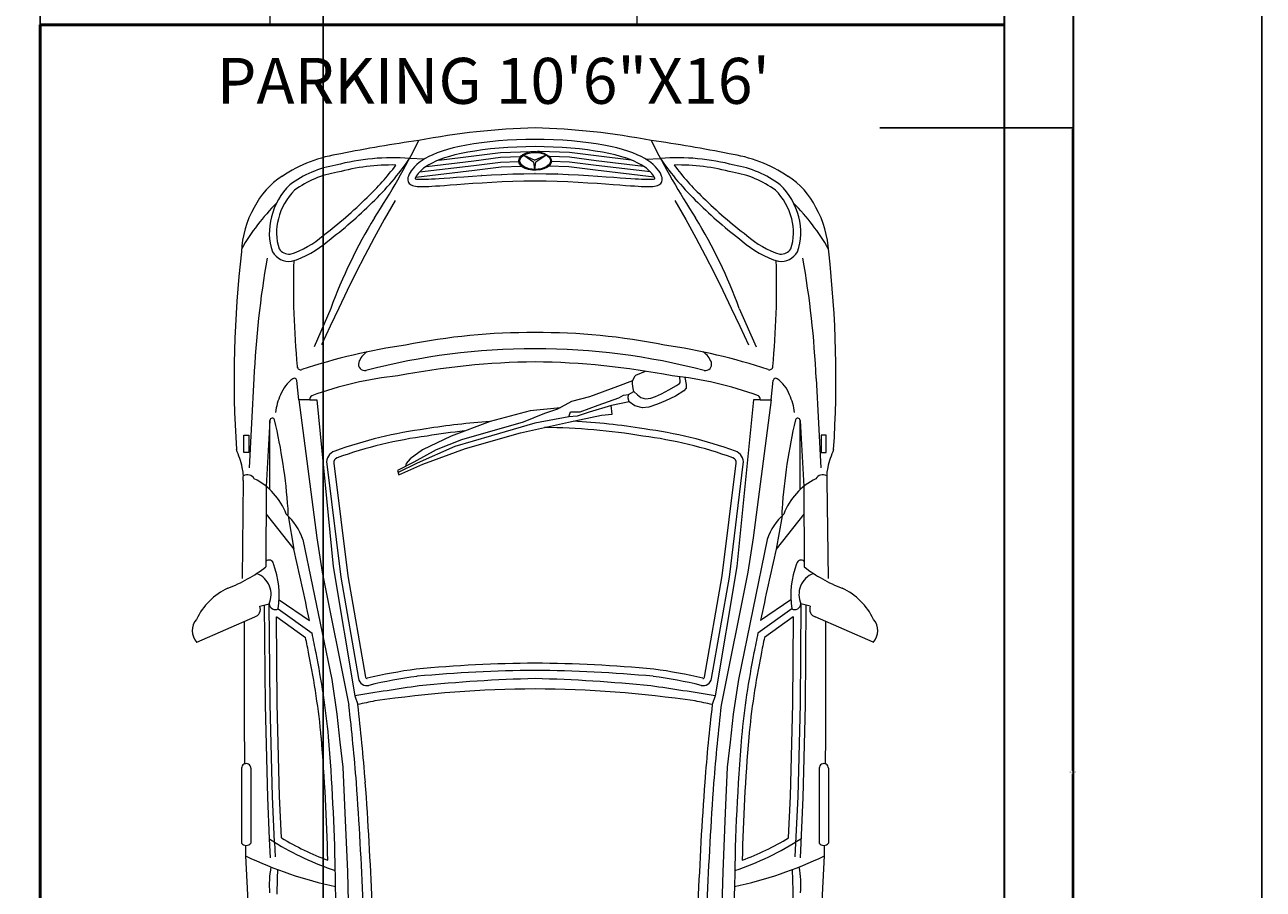
# Model space of a CAD drawing. Units: inches. Extents: x 8049 to 8459, y 820 to 1350.
# Tile 21 of 25: x 8297 to 8459, y 933 to 1046. Entities that reach past the tile are written whole.
import ezdxf

# ---------------------------------------------------------------- set-up
doc = ezdxf.new("R2010")
doc.units = ezdxf.units.IN
doc.header["$MEASUREMENT"] = 0
for name, color, linetype, lineweight in [('A-ANNO-DIMS', 2, 'Continuous', 18), ('A-AREA-IDEN', 7, 'Continuous', 25), ('A-GLAZ', 4, 'Continuous', 18), ('A-WALL', 7, 'Continuous', 50), ('C-PKNG-VEH', 8, 'Continuous', 13), ('C-SITE-WALL', 7, 'Continuous', 35)]:
    doc.layers.add(name, color=color, linetype=linetype, lineweight=lineweight)
doc.styles.get("Standard").update_dxf_attribs({"font": 'arial.ttf'})
doc.dimstyles.get("Standard").update_dxf_attribs({"dimtxt": 0.18, "dimasz": 0.18, "dimexe": 0.18, "dimexo": 0.0625, "dimgap": 0.09, "dimtad": 0, "dimtih": 1, "dimtoh": 1, "dimdec": 4, "dimzin": 0, "dimdsep": 46, "dimtxsty": 'Standard', "dimcen": 0.09, "dimadec": 0, "dimazin": 0, "dimtfac": 1, "dimtdec": 4, "dimtofl": 0, "dimtmove": 0, "dimatfit": 3, "dimfxl": 1, "dimtolj": 1, "dimtzin": 0, "dimarcsym": 0})

# ---------------------------------------------------------------- blocks, each defined once
blk = doc.blocks.new('A$C27D64469')
for p, q in [((-0.156, -0.4453), (-0.1764, -0.4487)), ((-0.1343, -0.4422), (-0.156, -0.4453)), ((-0.1114, -0.4395), (-0.1343, -0.4422)), ((-0.0875, -0.4373), (-0.1114, -0.4395)), ((-0.0629, -0.4354), (-0.0875, -0.4373)), ((-0.0377, -0.4341), (-0.0629, -0.4354)), ((-0.0122, -0.4333), (-0.0377, -0.4341)), ((0.0136, -0.433), (-0.0122, -0.4333)), ((0.0393, -0.4333), (0.0136, -0.433)), ((0.0649, -0.4341), (0.0393, -0.4333)), ((0.0901, -0.4354), (0.0649, -0.4341)), ((0.1147, -0.4373), (0.0901, -0.4354)), ((0.1385, -0.4395), (0.1147, -0.4373)), ((0.1614, -0.4422), (0.1385, -0.4395)), ((0.1832, -0.4453), (0.1614, -0.4422)), ((0.2036, -0.4487), (0.1832, -0.4453)), ((-0.2693, -0.4753), (-0.2803, -0.4806)), ((-0.2571, -0.4703), (-0.2693, -0.4753)), ((-0.2436, -0.4655), (-0.2571, -0.4703)), ((-0.253, -0.4902), (-0.1557, -0.4786)), ((-0.2289, -0.4609), (-0.2436, -0.4655)), ((-0.2128, -0.4566), (-0.2289, -0.4609)), ((-0.208, -0.476), (-0.2233, -0.4801)), ((-0.1954, -0.4525), (-0.2128, -0.4566)), ((-0.1912, -0.4721), (-0.208, -0.476)), ((-0.1764, -0.4487), (-0.1954, -0.4525)), ((-0.1728, -0.4684), (-0.1912, -0.4721)), ((-0.153, -0.4651), (-0.1728, -0.4684)), ((-0.1557, -0.4786), (-0.0819, -0.4693)), ((-0.1317, -0.4621), (-0.153, -0.4651)), ((-0.1093, -0.4594), (-0.1317, -0.4621)), ((-0.0858, -0.4572), (-0.1093, -0.4594)), ((-0.0616, -0.4554), (-0.0858, -0.4572)), ((-0.0819, -0.4693), (0.0012, -0.4665)), ((-0.0369, -0.4541), (-0.0616, -0.4554)), ((-0.0117, -0.4533), (-0.0369, -0.4541)), ((-0.0174, -0.4766), (0.0132, -0.4908)), ((-0.0174, -0.4766), (0.0101, -0.4961)), ((0.0136, -0.453), (-0.0117, -0.4533)), ((0.0012, -0.4665), (0.0067, -0.4665)), ((0.0445, -0.4762), (0.0132, -0.4908)), ((0.0389, -0.4533), (0.0136, -0.453)), ((0.0445, -0.4762), (0.0162, -0.4961)), ((0.0259, -0.4665), (0.0204, -0.4665)), ((0.109, -0.4693), (0.0259, -0.4665)), ((0.064, -0.4541), (0.0389, -0.4533)), ((0.0888, -0.4554), (0.064, -0.4541)), ((0.113, -0.4572), (0.0888, -0.4554)), ((0.1828, -0.4786), (0.109, -0.4693)), ((0.1364, -0.4594), (0.113, -0.4572)), ((0.1588, -0.4621), (0.1364, -0.4594)), ((0.1801, -0.4651), (0.1588, -0.4621)), ((0.2, -0.4684), (0.1801, -0.4651)), ((0.2801, -0.4902), (0.1828, -0.4786)), ((0.2183, -0.4721), (0.2, -0.4684)), ((0.2225, -0.4525), (0.2036, -0.4487)), ((0.2351, -0.476), (0.2183, -0.4721)), ((0.24, -0.4566), (0.2225, -0.4525)), ((0.2505, -0.4801), (0.2351, -0.476)), ((0.2561, -0.4609), (0.24, -0.4566)), ((0.2708, -0.4655), (0.2561, -0.4609)), ((0.2842, -0.4703), (0.2708, -0.4655)), ((0.2964, -0.4753), (0.2842, -0.4703)), ((0.3075, -0.4806), (0.2964, -0.4753)), ((-0.2923, -0.4873), (-0.3337, -0.4857)), ((-0.3248, -0.514), (-0.329, -0.5195)), ((-0.3198, -0.5085), (-0.3248, -0.514)), ((-0.3138, -0.5028), (-0.3198, -0.5085)), ((-0.307, -0.4972), (-0.3138, -0.5028)), ((-0.2991, -0.4915), (-0.307, -0.4972)), ((-0.306, -0.5231), (-0.1557, -0.5051)), ((-0.2947, -0.513), (-0.3006, -0.5178)), ((-0.2902, -0.486), (-0.2991, -0.4915)), ((-0.288, -0.5082), (-0.2947, -0.513)), ((-0.2803, -0.4806), (-0.2902, -0.486)), ((-0.2883, -0.5077), (-0.2883, -0.5077)), ((-0.2801, -0.5033), (-0.288, -0.5082)), ((-0.287, -0.5076), (-0.1557, -0.4919)), ((-0.2712, -0.4984), (-0.2801, -0.5033)), ((-0.2612, -0.4936), (-0.2712, -0.4984)), ((-0.2499, -0.489), (-0.2612, -0.4936)), ((-0.2373, -0.4844), (-0.2499, -0.489)), ((-0.2233, -0.4801), (-0.2373, -0.4844)), ((-0.1557, -0.4919), (-0.0819, -0.4825)), ((-0.1557, -0.5051), (-0.0819, -0.4958)), ((-0.154, -0.5181), (-0.0802, -0.5088)), ((-0.0819, -0.4825), (-0.0265, -0.4807)), ((-0.0819, -0.4958), (-0.0315, -0.4941)), ((-0.0802, -0.5088), (-0.0242, -0.5069)), ((0.0133, -0.5159), (0.0101, -0.4961)), ((0.0133, -0.5159), (0.0162, -0.4961)), ((0.1074, -0.5088), (0.0513, -0.5069)), ((0.109, -0.4825), (0.0537, -0.4807)), ((0.109, -0.4958), (0.0586, -0.4941)), ((0.1811, -0.5181), (0.1074, -0.5088)), ((0.1828, -0.4919), (0.109, -0.4825)), ((0.1828, -0.5051), (0.109, -0.4958)), ((0.3141, -0.5076), (0.1828, -0.4919)), ((0.3332, -0.5231), (0.1828, -0.5051)), ((0.2644, -0.4844), (0.2505, -0.4801)), ((0.277, -0.489), (0.2644, -0.4844)), ((0.2883, -0.4936), (0.277, -0.489)), ((0.2984, -0.4984), (0.2883, -0.4936)), ((0.3073, -0.5033), (0.2984, -0.4984)), ((0.3151, -0.5082), (0.3073, -0.5033)), ((0.3174, -0.486), (0.3075, -0.4806)), ((0.3219, -0.513), (0.3151, -0.5082)), ((0.3262, -0.4915), (0.3174, -0.486)), ((0.3195, -0.4873), (0.3609, -0.4857)), ((0.3277, -0.5178), (0.3219, -0.513)), ((0.3341, -0.4972), (0.3262, -0.4915)), ((0.341, -0.5028), (0.3341, -0.4972)), ((0.3469, -0.5085), (0.341, -0.5028)), ((0.352, -0.514), (0.3469, -0.5085)), ((0.3562, -0.5195), (0.352, -0.514)), ((-0.3381, -0.5386), (-0.3386, -0.5425)), ((-0.3386, -0.5425), (-0.3385, -0.5462)), ((-0.3385, -0.5462), (-0.3378, -0.5495)), ((-0.3369, -0.5343), (-0.3381, -0.5386)), ((-0.3351, -0.5296), (-0.3369, -0.5343)), ((-0.3324, -0.5247), (-0.3351, -0.5296)), ((-0.329, -0.5195), (-0.3324, -0.5247)), ((-0.318, -0.5407), (-0.3183, -0.5417)), ((-0.3183, -0.5417), (-0.3172, -0.542)), ((-0.3169, -0.5381), (-0.318, -0.5407)), ((-0.3172, -0.542), (-0.3144, -0.5426)), ((-0.3152, -0.5348), (-0.3169, -0.5381)), ((-0.3166, -0.5376), (-0.154, -0.5181)), ((-0.3127, -0.5311), (-0.3152, -0.5348)), ((-0.3144, -0.5426), (-0.3108, -0.543)), ((-0.3095, -0.5269), (-0.3127, -0.5311)), ((-0.3108, -0.543), (-0.3063, -0.5433)), ((-0.3055, -0.5225), (-0.3095, -0.5269)), ((-0.3063, -0.5433), (-0.3012, -0.5434)), ((-0.3006, -0.5178), (-0.3055, -0.5225)), ((-0.3012, -0.5434), (-0.2953, -0.5434)), ((-0.2953, -0.5434), (-0.2888, -0.5433)), ((-0.2888, -0.5433), (-0.2815, -0.543)), ((-0.2815, -0.543), (-0.2731, -0.5425)), ((-0.2731, -0.5425), (-0.2632, -0.5419)), ((-0.2632, -0.5419), (-0.2517, -0.5411)), ((-0.2517, -0.5411), (-0.2382, -0.5402)), ((-0.2382, -0.5402), (-0.2225, -0.539)), ((-0.2225, -0.539), (-0.2042, -0.5376)), ((-0.2042, -0.5376), (-0.1833, -0.5361)), ((-0.1832, -0.5361), (-0.1598, -0.5344)), ((-0.1597, -0.5344), (-0.1342, -0.5327)), ((-0.1341, -0.5327), (-0.1069, -0.5311)), ((-0.1067, -0.5311), (-0.0781, -0.5297)), ((-0.0779, -0.5297), (-0.0482, -0.5285)), ((-0.048, -0.5285), (-0.0176, -0.5278)), ((-0.0475, -0.5485), (-0.0171, -0.5478)), ((-0.0173, -0.5278), (0.0134, -0.5275)), ((-0.0171, -0.5478), (0.0136, -0.5475)), ((0.0136, -0.5475), (0.0443, -0.5478)), ((0.0138, -0.5275), (0.0444, -0.5278)), ((0.0443, -0.5478), (0.0746, -0.5485)), ((0.0448, -0.5278), (0.0751, -0.5285)), ((0.0754, -0.5285), (0.105, -0.5297)), ((0.1052, -0.5297), (0.1339, -0.5311)), ((0.134, -0.5311), (0.1612, -0.5327)), ((0.1614, -0.5327), (0.1869, -0.5344)), ((0.3438, -0.5376), (0.1811, -0.5181)), ((0.187, -0.5344), (0.2103, -0.5361)), ((0.2104, -0.5361), (0.2314, -0.5376)), ((0.2314, -0.5376), (0.2496, -0.539)), ((0.2496, -0.539), (0.2653, -0.5402)), ((0.2653, -0.5402), (0.2788, -0.5411)), ((0.2788, -0.5411), (0.2904, -0.5419)), ((0.2904, -0.5419), (0.3002, -0.5425)), ((0.3002, -0.5425), (0.3087, -0.543)), ((0.3087, -0.543), (0.316, -0.5433)), ((0.316, -0.5433), (0.3225, -0.5434)), ((0.3225, -0.5434), (0.3283, -0.5434)), ((0.3326, -0.5225), (0.3277, -0.5178)), ((0.3283, -0.5434), (0.3335, -0.5433)), ((0.3367, -0.5269), (0.3326, -0.5225)), ((0.3335, -0.5433), (0.3379, -0.543)), ((0.3399, -0.5311), (0.3367, -0.5269)), ((0.3379, -0.543), (0.3416, -0.5426)), ((0.3423, -0.5348), (0.3399, -0.5311)), ((0.3416, -0.5426), (0.3444, -0.542)), ((0.3441, -0.5381), (0.3423, -0.5348)), ((0.3451, -0.5407), (0.3441, -0.5381)), ((0.3444, -0.542), (0.3454, -0.5417)), ((0.3454, -0.5417), (0.3451, -0.5407)), ((0.3596, -0.5247), (0.3562, -0.5195)), ((0.3622, -0.5296), (0.3596, -0.5247)), ((0.3641, -0.5343), (0.3622, -0.5296)), ((0.3653, -0.5386), (0.3641, -0.5343)), ((0.3649, -0.5495), (0.3656, -0.5462)), ((0.3658, -0.5425), (0.3653, -0.5386)), ((0.3656, -0.5462), (0.3658, -0.5425)), ((-0.3378, -0.5495), (-0.3364, -0.5524)), ((-0.3364, -0.5524), (-0.3345, -0.5549)), ((-0.3345, -0.5549), (-0.3321, -0.5571)), ((-0.3321, -0.5571), (-0.3292, -0.5589)), ((-0.3292, -0.5589), (-0.3258, -0.5604)), ((-0.3258, -0.5604), (-0.3219, -0.5615)), ((-0.3219, -0.5615), (-0.3175, -0.5623)), ((-0.3175, -0.5623), (-0.3126, -0.5629)), ((-0.3126, -0.5629), (-0.3072, -0.5633)), ((-0.3072, -0.5633), (-0.3014, -0.5634)), ((-0.3014, -0.5634), (-0.2951, -0.5634)), ((-0.2951, -0.5634), (-0.2882, -0.5633)), ((-0.2882, -0.5633), (-0.2806, -0.563)), ((-0.2806, -0.563), (-0.272, -0.5625)), ((-0.272, -0.5625), (-0.2619, -0.5619)), ((-0.2619, -0.5619), (-0.2503, -0.5611)), ((-0.2503, -0.5611), (-0.2367, -0.5601)), ((-0.2367, -0.5601), (-0.221, -0.559)), ((-0.221, -0.559), (-0.2027, -0.5576)), ((-0.2027, -0.5576), (-0.1818, -0.556)), ((-0.1818, -0.556), (-0.1584, -0.5544)), ((-0.1584, -0.5544), (-0.1329, -0.5527)), ((-0.1329, -0.5527), (-0.1057, -0.5511)), ((-0.1057, -0.5511), (-0.0771, -0.5496)), ((-0.0771, -0.5496), (-0.0475, -0.5485)), ((0.0746, -0.5485), (0.1043, -0.5496)), ((0.1043, -0.5496), (0.1329, -0.5511)), ((0.1329, -0.5511), (0.1601, -0.5527)), ((0.1601, -0.5527), (0.1855, -0.5544)), ((0.1855, -0.5544), (0.2089, -0.556)), ((0.2089, -0.556), (0.2299, -0.5576)), ((0.2299, -0.5576), (0.2481, -0.559)), ((0.2481, -0.559), (0.2639, -0.5601)), ((0.2639, -0.5601), (0.2775, -0.5611)), ((0.2775, -0.5611), (0.2891, -0.5619)), ((0.2891, -0.5619), (0.2991, -0.5625)), ((0.2991, -0.5625), (0.3078, -0.563)), ((0.3078, -0.563), (0.3154, -0.5633)), ((0.3154, -0.5633), (0.3222, -0.5634)), ((0.3222, -0.5634), (0.3285, -0.5634)), ((0.3285, -0.5634), (0.3344, -0.5633)), ((0.3344, -0.5633), (0.3398, -0.5629)), ((0.3398, -0.5629), (0.3446, -0.5623)), ((0.3446, -0.5623), (0.349, -0.5615)), ((0.349, -0.5615), (0.3529, -0.5604)), ((0.3529, -0.5604), (0.3563, -0.5589)), ((0.3563, -0.5589), (0.3593, -0.5571)), ((0.3593, -0.5571), (0.3617, -0.5549)), ((0.3617, -0.5549), (0.3636, -0.5524)), ((0.3636, -0.5524), (0.3649, -0.5495)), ((-0.3736, -0.602), (-0.4036, -0.6546)), ((0.4008, -0.602), (0.4307, -0.6546)), ((-0.4036, -0.6546), (-0.4313, -0.7051)), ((0.4307, -0.6546), (0.4585, -0.7051)), ((-0.4313, -0.7051), (-0.4574, -0.7542)), ((0.4585, -0.7051), (0.4846, -0.7542)), ((-0.4574, -0.7542), (-0.4822, -0.8025)), ((0.4846, -0.7542), (0.5094, -0.8025)), ((-0.4822, -0.8025), (-0.5062, -0.8507)), ((0.5094, -0.8025), (0.5333, -0.8507)), ((-0.5062, -0.8507), (-0.5297, -0.8995)), ((0.5333, -0.8507), (0.5568, -0.8995)), ((-0.552, -0.901), (-0.5982, -1.0071)), ((-0.5297, -0.8995), (-0.5532, -0.9495)), ((0.5568, -0.8995), (0.5804, -0.9495)), ((0.5791, -0.901), (0.6253, -1.0071)), ((-0.5532, -0.9495), (-0.5772, -1.0014)), ((0.5804, -0.9495), (0.6044, -1.0014)), ((-0.7646, -1.0944), (-0.7774, -1.3418)), ((0.2832, -1.1011), (0.2905, -1.0871)), ((0.2925, -1.0852), (0.3197, -1.0743)), ((0.4151, -1.1035), (0.4148, -1.0897)), ((0.4283, -1.0915), (0.4315, -1.1115)), ((0.7917, -1.0944), (0.8046, -1.3418)), ((-0.6398, -1.1535), (-0.646, -1.0999)), ((0.2417, -1.1168), (0.1646, -1.1448)), ((0.2832, -1.1011), (0.2417, -1.1168)), ((0.2722, -1.1385), (0.2873, -1.1305)), ((0.283, -1.1095), (0.2832, -1.1011)), ((0.2848, -1.1224), (0.283, -1.1095)), ((0.2873, -1.1305), (0.2848, -1.1224)), ((0.2873, -1.1305), (0.2969, -1.1395)), ((0.3634, -1.137), (0.3841, -1.1257)), ((0.3841, -1.1257), (0.4048, -1.1143)), ((0.4254, -1.1287), (0.4022, -1.1436)), ((0.4048, -1.1143), (0.4131, -1.1088)), ((0.4131, -1.1088), (0.4151, -1.106)), ((0.4151, -1.106), (0.4151, -1.1035)), ((0.4315, -1.1216), (0.4254, -1.1287)), ((0.4315, -1.1115), (0.4315, -1.1216)), ((0.6669, -1.1535), (0.6731, -1.0999)), ((-0.6398, -1.1535), (-0.5904, -1.5351)), ((-0.61, -1.1535), (-0.6398, -1.1535)), ((-0.61, -1.1535), (-0.5908, -1.1535)), ((-0.5908, -1.1535), (-0.5454, -1.6151)), ((0.1143, -1.158), (0.0761, -1.1797)), ((0.1646, -1.1448), (0.1143, -1.158)), ((0.188, -1.1683), (0.2457, -1.1477)), ((0.2744, -1.1592), (0.2252, -1.1688)), ((0.2457, -1.1477), (0.2589, -1.1408)), ((0.2589, -1.1408), (0.2722, -1.1385)), ((0.2711, -1.1491), (0.2722, -1.1385)), ((0.2744, -1.1592), (0.2711, -1.1491)), ((0.2895, -1.1703), (0.2744, -1.1592)), ((0.2969, -1.1395), (0.3069, -1.1474)), ((0.3069, -1.1474), (0.3193, -1.1504)), ((0.3193, -1.1504), (0.3339, -1.1491)), ((0.3339, -1.1491), (0.3475, -1.1443)), ((0.3475, -1.1443), (0.3634, -1.137)), ((0.3745, -1.1567), (0.3526, -1.1658)), ((0.4022, -1.1436), (0.3745, -1.1567)), ((0.618, -1.1535), (0.5726, -1.6151)), ((0.6669, -1.1535), (0.6175, -1.5351)), ((0.6371, -1.1535), (0.618, -1.1535)), ((0.6371, -1.1535), (0.6669, -1.1535)), ((0, -1.1841), (-0.1108, -1.2136)), ((0.0401, -1.1917), (-0.0188, -1.2151)), ((0.0839, -1.1753), (0, -1.1841)), ((0.0761, -1.1797), (0.0401, -1.1917)), ((0.1062, -1.2154), (0.1972, -1.1964)), ((0.1069, -1.2008), (0.112, -1.1865)), ((0.1298, -1.1986), (0.1069, -1.2008)), ((0.112, -1.1865), (0.1383, -1.1871)), ((0.1635, -1.1877), (0.1298, -1.1986)), ((0.1383, -1.1871), (0.188, -1.1683)), ((0.2252, -1.1688), (0.1635, -1.1877)), ((0.1972, -1.1964), (0.2271, -1.1931)), ((0.2271, -1.1931), (0.2246, -1.169)), ((0.3107, -1.1759), (0.2895, -1.1703)), ((0.3289, -1.1738), (0.3107, -1.1759)), ((0.3526, -1.1658), (0.3289, -1.1738)), ((-0.7203, -1.2103), (-0.7302, -1.3933)), ((-0.7203, -1.4019), (-0.7203, -1.2103)), ((-0.1108, -1.2136), (-0.2189, -1.2538)), ((-0.0188, -1.2151), (-0.1903, -1.264)), ((0.013, -1.2184), (-0.1069, -1.2532)), ((-0.0266, -1.2451), (0.1062, -1.2154)), ((0.1069, -1.2008), (0.013, -1.2184)), ((0.7474, -1.4019), (0.7474, -1.2103)), ((0.7474, -1.2103), (0.7573, -1.3933)), ((-0.7922, -1.2996), (-0.7922, -1.251)), ((-0.7922, -1.251), (-0.7785, -1.251)), ((-0.7785, -1.251), (-0.7785, -1.2996)), ((-0.2189, -1.2538), (-0.2983, -1.2922)), ((-0.1903, -1.264), (-0.2605, -1.2919)), ((-0.1069, -1.2532), (-0.2084, -1.2823)), ((-0.1789, -1.2879), (-0.0266, -1.2451)), ((0.8056, -1.251), (0.8056, -1.2996)), ((0.8193, -1.251), (0.8056, -1.251)), ((0.8193, -1.2996), (0.8193, -1.251)), ((-0.7785, -1.2996), (-0.7922, -1.2996)), ((-0.2983, -1.2922), (-0.3323, -1.3172)), ((-0.2605, -1.2919), (-0.3222, -1.3262)), ((-0.2084, -1.2823), (-0.3128, -1.3287)), ((-0.2968, -1.3312), (-0.1789, -1.2879)), ((0.8056, -1.2996), (0.8193, -1.2996)), ((-0.563, -1.3311), (-0.5244, -1.6438)), ((-0.5431, -1.3287), (-0.5046, -1.6408)), ((-0.3222, -1.3262), (-0.3675, -1.3491)), ((-0.3128, -1.3287), (-0.3653, -1.355)), ((-0.363, -1.3611), (-0.2968, -1.3312)), ((-0.343, -1.3297), (-0.345, -1.3377)), ((-0.3323, -1.3172), (-0.343, -1.3297)), ((0.5317, -1.6408), (0.5703, -1.3287)), ((0.5515, -1.6438), (0.5901, -1.3311)), ((-0.3675, -1.3491), (-0.363, -1.3611)), ((-0.7946, -1.3764), (-0.7975, -1.6481)), ((-0.7302, -1.3933), (-0.7314, -1.6155)), ((0.7573, -1.3933), (0.7586, -1.6155)), ((0.8217, -1.3764), (0.8246, -1.6481)), ((-0.7306, -1.4695), (-0.6539, -1.5666)), ((0.7578, -1.4695), (0.681, -1.5666)), ((-0.6702, -1.4746), (-0.6539, -1.5666)), ((0.6973, -1.4746), (0.681, -1.5666)), ((-0.6294, -1.5396), (-0.5492, -1.9272)), ((-0.5904, -1.5351), (-0.5754, -1.6301)), ((0.6565, -1.5396), (0.5764, -1.9272)), ((0.6175, -1.5351), (0.6026, -1.6301)), ((-0.5754, -1.6301), (-0.5017, -1.9986)), ((-0.5454, -1.6151), (-0.4851, -1.9723)), ((-0.5244, -1.6438), (-0.475, -1.9247)), ((-0.5046, -1.6408), (-0.4553, -1.9213)), ((0.4824, -1.9213), (0.5317, -1.6408)), ((0.5021, -1.9247), (0.5515, -1.6438)), ((0.5726, -1.6151), (0.5122, -1.9723)), ((0.6026, -1.6301), (0.5289, -1.9986)), ((-0.6947, -1.7069), (-0.6109, -1.7637)), ((0.7218, -1.7069), (0.638, -1.7637)), ((-0.7483, -1.7248), (-0.7225, -1.7182)), ((-0.7364, -1.7217), (-0.7338, -1.998)), ((-0.7199, -1.9952), (-0.7225, -1.7182)), ((-0.6971, -1.7317), (-0.6035, -1.7992)), ((0.7242, -1.7317), (0.6307, -1.7992)), ((0.7496, -1.7182), (0.7471, -1.9952)), ((0.7755, -1.7248), (0.7496, -1.7182)), ((0.7635, -1.7217), (0.761, -1.998)), ((-0.9228, -1.8245), (-0.7622, -1.7543)), ((-0.6999, -1.9949), (-0.7021, -1.7537)), ((-0.7009, -1.7536), (-0.6216, -1.8108)), ((0.7281, -1.7536), (0.6487, -1.8108)), ((0.7271, -1.9949), (0.7293, -1.7537)), ((0.9499, -1.8245), (0.7893, -1.7543)), ((-0.5492, -1.9272), (-0.5351, -2.0233)), ((0.5764, -1.9272), (0.5623, -2.0233)), ((-0.4851, -1.9723), (-0.477, -1.9966)), ((0.5122, -1.9723), (0.5041, -1.9966)), ((-0.7338, -1.998), (-0.7273, -2.254)), ((-0.7134, -2.2512), (-0.7199, -1.9952)), ((-0.6934, -2.2505), (-0.6999, -1.9949)), ((0.7206, -2.2505), (0.7271, -1.9949)), ((0.7471, -1.9952), (0.7406, -2.2512)), ((0.761, -1.998), (0.7545, -2.254)), ((-0.5351, -2.0233), (-0.5266, -2.1005)), ((0.5623, -2.0233), (0.5538, -2.1005)), ((-0.5266, -2.1005), (-0.5182, -2.1702)), ((0.5538, -2.1005), (0.5453, -2.1702)), ((-0.7987, -2.1729), (-0.7987, -2.3802)), ((-0.7732, -2.1729), (-0.7732, -2.3802)), ((-0.5182, -2.1702), (-0.5125, -2.2965)), ((0.5453, -2.1702), (0.5397, -2.2965)), ((0.8003, -2.1729), (0.8003, -2.3802)), ((0.8259, -2.1729), (0.8259, -2.3802)), ((-0.7273, -2.254), (-0.7223, -2.368)), ((-0.7078, -2.3771), (-0.7134, -2.2512)), ((-0.6883, -2.3655), (-0.6934, -2.2505)), ((0.7155, -2.3655), (0.7206, -2.2505)), ((0.7406, -2.2512), (0.7332, -2.4181)), ((0.7545, -2.254), (0.7471, -2.4209)), ((-0.5125, -2.2965), (-0.5059, -2.4594)), ((0.5397, -2.2965), (0.5331, -2.4594)), ((-0.7223, -2.368), (-0.7199, -2.4209)), ((-0.7078, -2.3771), (-0.706, -2.4181)), ((-0.5059, -2.4594), (-0.4945, -2.8747)), ((0.5331, -2.4594), (0.5216, -2.8747))]:
    blk.add_line(p, q)
for centre, radius, start, end in [((0.0637, -2.359), 1.9586, 91.468, 100.9476), ((-0.0366, -2.359), 1.9586, 79.0524, 88.532), ((0.1265, -3.625), 3.2185, 97.7633, 101.6634), ((-2.1519, 0.4791), 2.0583, 326.7435, 333.6014), ((-0.0994, -3.625), 3.2185, 78.3366, 82.2367), ((2.179, 0.4791), 2.0583, 206.3986, 213.2565), ((-0.471, -0.8549), 0.3855, 97.9189, 123.9683), ((0.4981, -0.8549), 0.3855, 56.0317, 82.0811), ((-0.4915, -0.79), 0.2893, 99.1695, 126.8677), ((-0.3813, -1.088), 0.6042, 85.4848, 104.9936), ((-0.3813, -1.088), 0.5842, 89.0187, 105.0943), ((-0.9467, -0.0711), 0.72, 313.4908, 323.0478), ((-0.9467, -0.0711), 0.74, 313.509, 325.9238), ((0.4084, -1.088), 0.6042, 75.0064, 94.5152), ((0.9738, -0.0711), 0.74, 214.0762, 226.491), ((0.4084, -1.088), 0.5842, 74.9057, 90.9813), ((0.9738, -0.0711), 0.72, 216.9522, 226.5092), ((0.5186, -0.79), 0.2893, 53.1323, 80.8305), ((-0.5677, -0.7201), 0.2198, 122.6776, 153.2639), ((-0.4915, -0.79), 0.2693, 98.9551, 126.5901), ((-0.2027, -0.5576), 0.02, 94.2621, 94.2814), ((-0.1818, -0.556), 0.02, 94.094, 94.2621), ((-0.1584, -0.5544), 0.02, 93.7902, 94.094), ((-0.1329, -0.5527), 0.02, 93.3698, 93.7902), ((-0.1057, -0.5511), 0.02, 92.8387, 93.3698), ((-0.0771, -0.5496), 0.02, 92.1933, 92.8387), ((-0.0475, -0.5485), 0.02, 91.423, 92.1933), ((-0.0171, -0.5478), 0.02, 90.5101, 91.423), ((0.0136, -0.5475), 0.02, 89.4899, 90.5101), ((0.0443, -0.5478), 0.02, 88.577, 89.4899), ((0.0746, -0.5485), 0.02, 87.8067, 88.577), ((0.1043, -0.5496), 0.02, 87.1613, 87.8067), ((0.1329, -0.5511), 0.02, 86.6302, 87.1613), ((0.1601, -0.5527), 0.02, 86.2098, 86.6302), ((0.1855, -0.5544), 0.02, 85.906, 86.2098), ((0.2089, -0.556), 0.02, 85.7379, 85.906), ((0.2299, -0.5576), 0.02, 85.7186, 85.7379), ((0.5186, -0.79), 0.2693, 53.4099, 81.0449), ((0.5949, -0.7201), 0.2198, 26.7361, 57.3224), ((-0.5339, -0.6931), 0.1879, 134.257, 165.9979), ((-0.5339, -0.6931), 0.1679, 134.6933, 166.0746), ((0.5611, -0.6931), 0.1679, 13.9254, 45.3067), ((0.5611, -0.6931), 0.1879, 14.0021, 45.743), ((-0.2571, -1.0501), 0.6264, 135.2689, 149.8576), ((-1.2622, 0.2224), 1.1505, 306.8088, 314.8317), ((-1.2622, 0.2224), 1.1705, 306.853, 314.8203), ((1.2894, 0.2224), 1.1705, 225.1797, 233.147), ((1.2894, 0.2224), 1.1505, 225.1683, 233.1912), ((0.2842, -1.0501), 0.6264, 30.1424, 44.7311), ((-0.5196, -0.7579), 0.2801, 150.7841, 177.1611), ((-0.5599, -0.6904), 0.1621, 164.7178, 199.3716), ((0.7633, -1.3808), 1.4001, 148.5187, 159.9579), ((-0.7362, -1.3808), 1.4001, 20.0421, 31.4813), ((0.587, -0.6904), 0.1621, 340.6284, 15.2822), ((0.5467, -0.7579), 0.2801, 2.8389, 29.2159), ((-0.5599, -0.6904), 0.1421, 164.6281, 198.5509), ((0.587, -0.6904), 0.1421, 341.4491, 15.3719), ((-0.7354, -0.5187), 0.2425, 286.9921, 312.0664), ((-0.7354, -0.5187), 0.2625, 286.5483, 311.8628), ((0.7625, -0.5187), 0.2625, 228.1372, 253.4517), ((0.7625, -0.5187), 0.2425, 227.9336, 253.0079), ((2.2292, -1.0935), 3.0486, 173.4174, 183.7163), ((-0.6669, -0.7176), 0.053, 210.0698, 276.7845), ((-0.6669, -0.7176), 0.033, 213.0457, 274.1097), ((0.694, -0.7176), 0.053, 263.2155, 329.9302), ((0.694, -0.7176), 0.033, 265.8903, 326.9543), ((-2.2021, -1.0935), 3.0486, 356.2837, 6.5826), ((1.7769, -1.2069), 2.544, 169.9235, 177.4667), ((1.7667, -0.8364), 2.422, 178.3888, 185.3284), ((-1.7396, -0.8364), 2.422, 354.6716, 1.6112), ((-1.7498, -1.2069), 2.544, 2.5333, 10.0765), ((0.0046, -2.7444), 1.777, 89.7096, 101.339), ((0.0226, -2.7444), 1.777, 78.661, 90.2904), ((-0.1068, -2.6471), 1.6622, 98.2339, 108.4059), ((-0.4223, -1.0677), 0.055, 122.1615, 161.7809), ((0.0163, -2.8903), 1.8782, 90.0843, 104.512), ((0.0108, -2.8903), 1.8782, 75.488, 89.9157), ((0.1339, -2.6471), 1.6622, 71.5941, 81.7661), ((0.4494, -1.0677), 0.055, 18.2191, 57.8385), ((-0.6348, -1.0604), 0.0101, 185.3284, 288.4059), ((-0.4585, -1.0557), 0.0168, 161.7809, 284.512), ((0.0393, -3.1787), 2.1304, 90.6925, 100.9626), ((-0.0122, -3.1787), 2.1304, 79.0374, 89.3075), ((0.4857, -1.0557), 0.0168, 255.488, 18.2191), ((0.6619, -1.0604), 0.0101, 251.5941, 354.6716), ((-0.6033, -1.1719), 0.0933, 124.7249, 159.8848), ((-0.6527, -1.1007), 0.00673, 6.5512, 124.7249), ((-0.2611, -2.0848), 1.0031, 95.9948, 110.0315), ((0.294, -1.0889), 0.004, 111.8862, 152.6845), ((0.2882, -2.0848), 1.0031, 69.9685, 84.0052), ((0.6798, -1.1007), 0.00673, 55.2751, 173.4488), ((0.6305, -1.1719), 0.0933, 20.1152, 55.2751), ((-0.5552, -1.2042), 0.1503, 154.6022, 174.0364), ((-0.5998, -1.1515), 0.0104, 118.0528, 191.1071), ((0.6269, -1.1515), 0.0104, 348.8929, 61.9472), ((0.5823, -1.2042), 0.1503, 5.9636, 25.3978), ((-0.7137, -1.2111), 0.00665, 15.5251, 172.9634), ((-2.218, -1.5637), 1.5518, 4.0302, 13.202), ((-0.1308, -2.4351), 1.2114, 97.4669, 109.7935), ((0.0017, -2.9892), 1.779, 93.6503, 99.3781), ((0.0254, -2.9892), 1.759, 80.6111, 89.5421), ((0.0254, -2.9892), 1.779, 80.6219, 86.9829), ((0.1579, -2.4351), 1.2114, 70.2065, 82.5331), ((2.2452, -1.5637), 1.5518, 166.798, 175.9698), ((0.7408, -1.2111), 0.00665, 7.0366, 164.4749), ((-0.1308, -2.4351), 1.1914, 97.4508, 109.7935), ((0.0017, -2.9892), 1.759, 95.9707, 99.3889), ((0.1579, -2.4351), 1.1914, 70.2065, 82.5492), ((-1.1013, -1.4136), 0.3132, 13.4845, 23.0084), ((-0.5296, -1.327), 0.0337, 109.7935, 187.0357), ((0.5567, -1.327), 0.0337, 352.9643, 70.2065), ((1.1284, -1.4136), 0.3132, 156.9916, 166.5155), ((-0.5296, -1.327), 0.0137, 109.7935, 187.0357), ((0.5567, -1.327), 0.0137, 352.9643, 70.2065), ((-0.8898, -1.3641), 0.096, 352.6385, 14.2173), ((-0.7831, -1.3832), 0.0225, 29.7837, 118.4161), ((0.8102, -1.3832), 0.0225, 61.5839, 150.2163), ((0.9169, -1.3641), 0.096, 165.7827, 187.3615), ((-0.8418, -1.5314), 0.1776, 20.2536, 63.8557), ((0.8689, -1.5314), 0.1776, 116.1443, 159.7464), ((-0.7826, -1.5905), 0.1615, 18.3646, 48.2784), ((-0.771, -1.4642), 0.1013, 354.1028, 5.3715), ((0.8098, -1.5905), 0.1615, 131.7216, 161.6354), ((0.7981, -1.4642), 0.1013, 174.6285, 185.8972), ((-10.825, -3.8887), 10.4328, 11.75206, 12.86028), ((10.8521, -3.8887), 10.4328, 167.13972, 168.24794), ((-0.7227, -1.6094), 0.0124, 11.3416, 134.5987), ((-0.9441, -1.6953), 0.2497, 351.6082, 20.7105), ((0.9712, -1.6953), 0.2497, 159.2895, 188.3918), ((0.7498, -1.6094), 0.0124, 45.4013, 168.6584), ((-0.9818, -1.2945), 0.4071, 290.8732, 307.9458), ((-0.7801, -1.6924), 0.0631, 335.8522, 68.2516), ((0.8072, -1.6924), 0.0631, 111.7484, 204.1478), ((1.0089, -1.2945), 0.4071, 232.0542, 249.1268), ((-0.7607, -1.8385), 0.1804, 114.9135, 154.5523), ((0.7879, -1.8385), 0.1804, 25.4477, 65.0865), ((-0.7685, -1.7333), 0.0219, 286.784, 22.9417), ((-0.7054, -1.7168), 0.0171, 184.6651, 299.1967), ((0.7326, -1.7168), 0.0171, 240.8033, 355.3349), ((0.7957, -1.7333), 0.0219, 157.0583, 253.216), ((-0.8877, -1.7923), 0.0477, 138.9599, 222.5475), ((28.5723, -1.9291), 29.3639, 179.68363, 180.45247), ((-0.7054, -1.7168), 0.0371, 275.0842, 276.9824), ((0.7326, -1.7168), 0.0371, 263.0176, 264.9158), ((-28.5452, -1.9291), 29.3639, 359.54753, 0.31637), ((0.9148, -1.7923), 0.0477, 317.4525, 41.0401), ((-10.825, -3.8887), 10.4128, 11.24635, 11.51036), ((-10.825, -3.8887), 10.4328, 11.24656, 11.5533), ((10.8521, -3.8887), 10.4328, 168.4467, 168.75344), ((10.8521, -3.8887), 10.4128, 168.48964, 168.75365), ((-2.7812, -2.2979), 2.2132, 5.4405, 11.4681), ((-2.7812, -2.2979), 2.2332, 5.4374, 11.4671), ((0.034, -5.6085), 3.7262, 90.3146, 95.3817), ((-0.0069, -5.6085), 3.7262, 84.6183, 89.6854), ((2.8083, -2.2979), 2.2332, 168.5329, 174.5626), ((2.8083, -2.2979), 2.2132, 168.5319, 174.5595), ((-0.1284, -3.2729), 1.3868, 97.7498, 103.4471), ((-0.1284, -3.2729), 1.3668, 97.7671, 103.4471), ((0.034, -5.6085), 3.7062, 90.3163, 95.3753), ((-0.0069, -5.6085), 3.7062, 84.6247, 89.6837), ((0.1556, -3.2729), 1.3668, 76.5529, 82.2329), ((0.1556, -3.2729), 1.3868, 76.5529, 82.2502), ((2.8455, -23.0231), 21.3127, 98.50598, 98.99062), ((-0.4518, -1.9207), 0.0236, 189.9743, 283.4471), ((-0.4518, -1.9207), 0.00357, 189.9743, 283.4471), ((0.0355, -5.2091), 3.2558, 90.3851, 98.2136), ((0.1214, -6.2334), 4.3098, 91.434, 95.7038), ((-0.0943, -6.2334), 4.3098, 84.2962, 88.566), ((-0.0083, -5.2091), 3.2558, 81.7864, 89.6149), ((-2.8184, -23.0231), 21.3127, 81.00938, 81.49402), ((0.4789, -1.9207), 0.0236, 256.5529, 350.0257), ((0.4789, -1.9207), 0.00357, 256.5529, 350.0257), ((-0.0958, -3.6836), 1.7295, 101.1311, 102.7329), ((0.1229, -3.6836), 1.7295, 77.2671, 78.8689), ((-6.4408, -2.6841), 5.9785, 4.51893, 6.58421), ((-6.416, -2.6821), 5.9785, 4.51893, 6.58421), ((6.4432, -2.6821), 5.9785, 173.41579, 175.48107), ((6.4679, -2.6841), 5.9785, 173.41579, 175.48107), ((-6.2705, -2.56), 5.7121, 1.3286, 4.7387), ((-6.2705, -2.56), 5.7321, 1.03863, 4.73991), ((6.2976, -2.56), 5.7321, 175.26009, 179.33379), ((6.2976, -2.56), 5.7121, 175.2613, 178.6714), ((-0.7859, -2.1729), 0.0128, 359.8097, 180.1903), ((0.8131, -2.1729), 0.0128, 359.8097, 180.1903), ((-11.1621, -2.9794), 10.7086, 2.32274, 4.10377), ((-11.1373, -2.9775), 10.7086, 2.32274, 4.10377), ((11.1645, -2.9775), 10.7086, 175.89623, 177.67726), ((11.1892, -2.9794), 10.7086, 175.89623, 177.67726), ((-0.7859, -2.3704), 0.0161, 217.6419, 322.3581), ((28.5723, -1.9291), 29.3639, 180.89229, 180.9487), ((-0.2816, -1.6867), 0.8114, 237.1024, 238.3082), ((-0.2816, -1.6867), 0.8114, 238.3082, 251.4793), ((-0.2816, -1.6867), 0.7914, 239.0709, 249.4088), ((0.3087, -1.6867), 0.8114, 288.5207, 302.8976), ((0.3087, -1.6867), 0.7914, 290.5912, 300.9291), ((0.8131, -2.3704), 0.0161, 217.6419, 322.3581), ((-28.5452, -1.9291), 29.3639, 359.0513, 359.10771), ((145.5619, 4.7984), 146.5271, 182.82189, 183.047472), ((-0.3074, -1.4152), 1.1094, 244.3519, 257.9711), ((0.3345, -1.4152), 1.1094, 282.0289, 295.6481), ((-145.5348, 4.7984), 146.5271, 356.952528, 357.17811), ((-0.4463, -2.4963), 0.2758, 169.4971, 184.519), ((2.1845, -2.5566), 2.8858, 177.9428, 179.2929), ((-6.2705, -2.56), 5.7321, 0.66621, 1.03863), ((-2.1573, -2.5566), 2.8858, 352.6735, 2.0572), ((0.4735, -2.4963), 0.2758, 355.481, 10.5029), ((-21.144, -3.0635), 20.6131, 1.44842, 1.58522), ((21.1711, -3.0635), 20.6131, 178.41478, 180.12035)]:
    blk.add_arc(centre, radius, start, end)
blk.add_ellipse((0.014, -0.4925), major_axis=(-0.0426, 0), ratio=0.550187)
blk.add_open_spline([(-0.0315, -0.4925), (-0.0315, -0.5012), (-0.0242, -0.5089), (0.0098, -0.5237), (0.0496, -0.5174), (0.0659, -0.4821), (0.0357, -0.4635), (-0.0133, -0.4686), (-0.0315, -0.4789), (-0.0315, -0.4925)], degree=3, knots=[0, 0, 0, 0, 0.903923, 0.903923, 2.878844, 2.878844, 4.872977, 4.872977, 6.283185, 6.283185, 6.283185, 6.283185])
blk = doc.blocks.new('WIN-48IN-SURROUND')
for p, q in [((9, 48), (0, 48)), ((0, 48), (0, 0)), ((0, 0), (9, 0))]:
    blk.add_line(p, q)
blk = doc.blocks.new('*D46')
at = {"layer": 'A-ANNO-DIMS', "color": 0, "lineweight": -2, "transparency": 16777216}
for p, q in [((8409.11, 1032.41), (8434.48, 1032.41)), ((8434.3, 1032.23), (8434.3, 948.43)), ((8434.3, 864.26), (8434.3, 948.06)), ((8409.11, 864.08), (8434.48, 864.08))]:
    blk.add_line(p, q, dxfattribs=at)
at = {"layer": 'A-ANNO-DIMS', "color": 0, "transparency": 16777216}
for points in [[(8434.27, 1032.23), (8434.33, 1032.23), (8434.3, 1032.41)], [(8434.27, 864.26), (8434.33, 864.26), (8434.3, 864.08)]]:
    blk.add_solid(points, dxfattribs=at)
at = {"layer": 'Defpoints', "color": 0, "transparency": 16777216}
for p in [(8409.05, 1032.41), (8434.3, 1032.41), (8409.05, 864.08)]:
    blk.add_point(p, dxfattribs=at)
at = {"layer": 'A-ANNO-DIMS', "color": 0, "transparency": 16777216, "insert": (8434.3, 948.24), "char_height": 0.18, "attachment_point": 5}
blk.add_mtext('\\A1;CAR 168', dxfattribs=at)
blk = doc.blocks.new('*D49')
at = {"layer": 'A-ANNO-DIMS', "color": 0, "lineweight": -2, "transparency": 16777216}
for p, q in [((8434.46, 1324.87), (8459.18, 1324.87)), ((8459, 1324.69), (8459, 1085.05)), ((8459, 845.05), (8459, 1084.69)), ((8434.46, 844.87), (8459.18, 844.87))]:
    blk.add_line(p, q, dxfattribs=at)
at = {"layer": 'A-ANNO-DIMS', "color": 0, "transparency": 16777216}
for points in [[(8458.97, 1324.69), (8459.03, 1324.69), (8459, 1324.87)], [(8458.97, 845.05), (8459.03, 845.05), (8459, 844.87)]]:
    blk.add_solid(points, dxfattribs=at)
at = {"layer": 'Defpoints', "color": 0, "transparency": 16777216}
for p in [(8434.4, 1324.87), (8459, 1324.87), (8434.4, 844.87)]:
    blk.add_point(p, dxfattribs=at)
at = {"layer": 'A-ANNO-DIMS', "color": 0, "transparency": 16777216, "insert": (8459, 1084.87), "char_height": 0.18, "attachment_point": 5}
blk.add_mtext('\\A1;480', dxfattribs=at)
blk = doc.blocks.new('*D66')
at = {"layer": 'A-ANNO-DIMS', "color": 0, "lineweight": -2, "transparency": 16777216}
for p, q in [((8336.4, 1267.81), (8336.4, 820.09)), ((8299.4, 1258.81), (8299.4, 820.09)), ((8299.58, 820.27), (8317.68, 820.27)), ((8336.22, 820.27), (8318.12, 820.27))]:
    blk.add_line(p, q, dxfattribs=at)
at = {"layer": 'A-ANNO-DIMS', "color": 0, "transparency": 16777216}
for points in [[(8299.58, 820.3), (8299.58, 820.24), (8299.4, 820.27)], [(8336.22, 820.3), (8336.22, 820.24), (8336.4, 820.27)]]:
    blk.add_solid(points, dxfattribs=at)
at = {"layer": 'Defpoints', "color": 0, "transparency": 16777216}
for p in [(8336.4, 1267.87), (8299.4, 1258.87), (8299.4, 820.27)]:
    blk.add_point(p, dxfattribs=at)
at = {"layer": 'A-ANNO-DIMS', "color": 0, "transparency": 16777216, "insert": (8317.9, 820.27), "char_height": 0.18, "attachment_point": 5}
blk.add_mtext('\\A1;37', dxfattribs=at)
blk = doc.blocks.new('*D76')
at = {"layer": 'A-ANNO-DIMS', "color": 0, "lineweight": -2, "transparency": 16777216}
for p, q in [((8083.4, 1054.81), (8083.4, 820.09)), ((8299.4, 1054.81), (8299.4, 820.09)), ((8083.58, 820.27), (8191.11, 820.27)), ((8299.22, 820.27), (8191.69, 820.27))]:
    blk.add_line(p, q, dxfattribs=at)
at = {"layer": 'A-ANNO-DIMS', "color": 0, "transparency": 16777216}
for points in [[(8083.58, 820.3), (8083.58, 820.24), (8083.4, 820.27)], [(8299.22, 820.3), (8299.22, 820.24), (8299.4, 820.27)]]:
    blk.add_solid(points, dxfattribs=at)
at = {"layer": 'Defpoints', "color": 0, "transparency": 16777216}
for p in [(8083.4, 1054.87), (8299.4, 1054.87), (8299.4, 820.27)]:
    blk.add_point(p, dxfattribs=at)
at = {"layer": 'A-ANNO-DIMS', "color": 0, "transparency": 16777216, "insert": (8191.4, 820.27), "char_height": 0.18, "attachment_point": 5}
blk.add_mtext('\\A1;216', dxfattribs=at)

msp = doc.modelspace()

# ---------------------------------------------------------------- linework, layer by layer
at = {"layer": 'A-WALL'}
for p, q in [((8299.3974, 853.8706), (8299.3974, 1045.8706)), ((8299.3974, 1045.8706), (8425.3974, 1045.8706))]:
    msp.add_line(p, q, dxfattribs=at)
at = {"layer": 'C-SITE-WALL'}
for p, q in [((8434.3974, 844.8706), (8434.3974, 1324.8706)), ((8425.3974, 853.8706), (8425.3974, 1315.8706))]:
    msp.add_line(p, q, dxfattribs=at)

# ---------------------------------------------------------------- block references
at = {"layer": 'A-GLAZ', "rotation": 89.99999999999795}
msp.add_blockref('WIN-48IN-SURROUND', (8377.397, 1045.8702), dxfattribs=at)
at = {"layer": 'C-PKNG-VEH', "xscale": 47.19862401584114, "yscale": 47.19862401584114, "zscale": 47.19862401584114}
msp.add_blockref('A$C27D64469', (8363.4216, 1051.3375), dxfattribs=at)

# ---------------------------------------------------------------- texts
at = {"layer": 'A-AREA-IDEN'}
msp.add_text('PARKING 10\'6"X16\'', height=6, dxfattribs=at).set_placement((8322.4849, 1035.5481))

# ---------------------------------------------------------------- dimensions: what is measured, and where the dimension line sits
at = {"layer": 'A-ANNO-DIMS'}
dim = msp.add_linear_dim(base=(8458.9974, 1324.8706), p1=(8434.3974, 844.8706), p2=(8434.3974, 1324.8706), angle=90, dimstyle='Standard', override={"dimdec": 0, "dimlfac": 1, "dimrnd": 0, "dimzin": 0, "dimdsep": 46, "dimlunit": 2}, dxfattribs=at)
dim.commit()
dim.dimension.update_dxf_attribs({"geometry": '*D49', "text_midpoint": (8458.9974, 1084.8706)})
for p1, p2, picture, middle in [((8336.3974, 1267.8706), (8299.3974, 1258.8706), '*D66', (8317.8974, 820.2706)), ((8083.3974, 1054.8706), (8299.3974, 1054.8706), '*D76', (8191.3974, 820.2706))]:
    dim = msp.add_linear_dim(base=(8299.3974, 820.2706), p1=p1, p2=p2, dimstyle='Standard', override={"dimdec": 0, "dimlfac": 1, "dimrnd": 0, "dimzin": 0, "dimdsep": 46, "dimlunit": 2}, dxfattribs=at)
    dim.commit()
    dim.dimension.update_dxf_attribs({"geometry": picture, "text_midpoint": middle})
dim = msp.add_linear_dim(base=(8434.2984, 1032.4086), p1=(8409.0493, 864.0808), p2=(8409.0493, 1032.4086), angle=90, text='CAR <>', dimstyle='Standard', override={"dimdec": 0, "dimlfac": 1, "dimrnd": 0, "dimzin": 0, "dimdsep": 46, "dimlunit": 2}, dxfattribs=at)
dim.commit()
dim.dimension.update_dxf_attribs({"geometry": '*D46', "text_midpoint": (8434.2984, 948.2447)})

doc.saveas('drawing.dxf')
